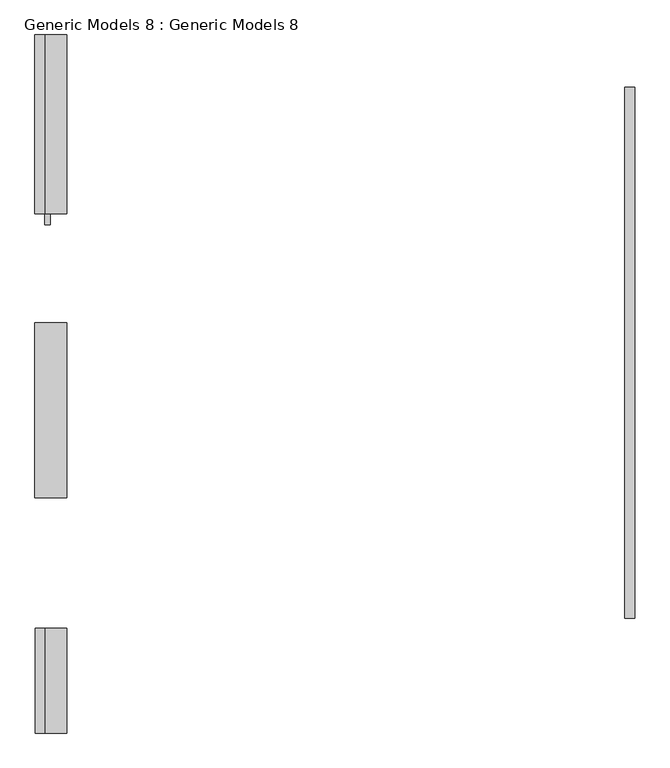
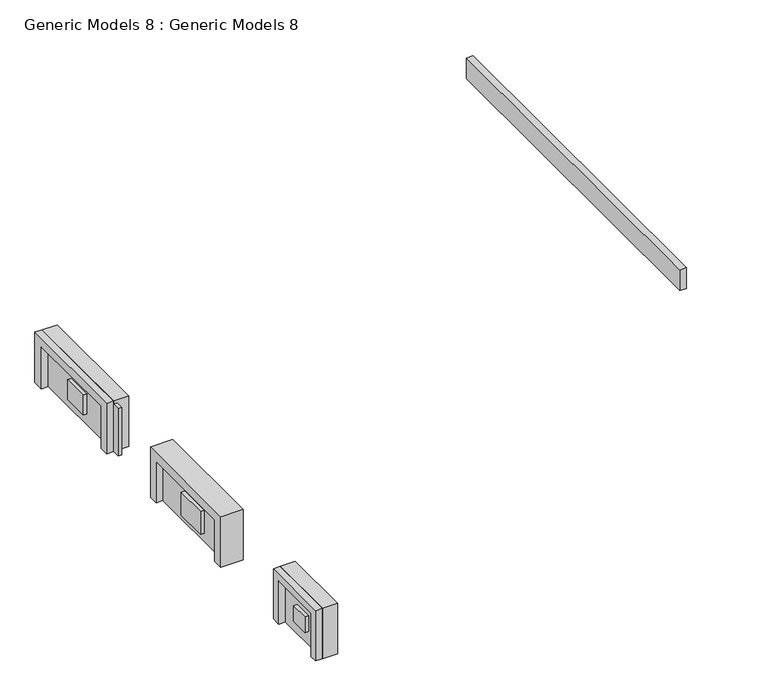
"""IFC4 building model written with IfcOpenShell, lengths in millimetres: proxy geometry, Generic Models 8 : Generic Models 8."""

from ifc_helpers import new_model, si_unit, frame, origin, origin_with_axes, place, context, project, spatial, polyline, outline, extrude, faceted_brep, source, transform, mapped, element, save


def generic_models_8_generic_models_8_478b8fa0(model_context):
    return source(origin(), model_context, "Body", "SolidModel", [
        extrude(outline(polyline([(-7844.1503587, -13644.7526331), (-7844.1503587, -1224.1526331), (-7615.5503587, -1224.1526331), (-7615.5503587, -13644.7526331), (-7844.1503587, -13644.7526331)])), frame((0.0, 0.0, 6400.8), z_axis=(0.0, 0.0, 1.0), x_axis=(1.0, 0.0, 0.0)), (0.0, 0.0, 1.0), 737.5181991),
        extrude(outline(polyline([(-21535.9206529, -15534.9751269), (-21535.9206529, -14874.5751269), (-21408.9206529, -14874.5751269), (-21408.9206529, -15534.9751269), (-21535.9206529, -15534.9751269)])), frame((0.0, 0.0, 181.195359), z_axis=(0.0, 0.0, 1.0), x_axis=(1.0, 0.0, 0.0)), (0.0, 0.0, 1.0), 558.8),
        extrude(outline(polyline([(-13873.3526331, -304.8), (-14178.4839562, -304.8), (-14178.4839562, 1232.1316532), (-16074.0892499, 1232.1316532), (-16074.0892499, -304.8), (-16330.8026331, -304.8), (-16330.8026331, 1483.4369838), (-13873.3526331, 1483.4369838), (-13873.3526331, -304.8)])), frame((-21637.5206529, 0.0, 0.0), z_axis=(1.0, 0.0, 0.0), x_axis=(0.0, 1.0, 0.0)), (0.0, 0.0, 1.0), 228.6),
        extrude(outline(polyline([(-21543.2828462, -9472.8026331), (-21543.2828462, -8342.5026331), (-21416.2828462, -8342.5026331), (-21416.2828462, -9472.8026331), (-21543.2828462, -9472.8026331)])), origin_with_axes(), (0.0, 0.0, 1.0), 812.6731894),
        faceted_brep([(-21644.8828462, -6729.6026331, -304.8), (-21644.8828462, -7051.784928, -304.8), (-21644.8828462, -7051.784928, 1165.4262933), (-21644.8828462, -10472.6342949, 1165.4262933), (-21644.8828462, -10472.6342949, -304.8), (-21644.8828462, -10825.3526331, -304.8), (-21644.8828462, -10825.3526331, 1483.4369838), (-21644.8828462, -6729.6026331, 1483.4369838), (-20900.9206529, -6729.6026331, -304.8), (-20900.9206529, -10825.3526331, -304.8), (-21416.2828462, -10472.6342949, -304.8), (-21416.2828462, -7051.784928, -304.8), (-21416.2828462, -7051.784928, 1165.4262933), (-20900.9206529, -10825.3526331, 1483.4369838), (-20900.9206529, -6729.6026331, 1483.4369838), (-21416.2828462, -10472.6342949, 1165.4262933)], [[[0, 1, 2, 3, 4, 5, 6, 7]], [[1, 0, 8, 9, 5, 4, 10, 11]], [[2, 1, 11, 12]], [[7, 6, 13, 14]], [[0, 7, 14, 8]], [[3, 2, 12, 15]], [[6, 5, 9, 13]], [[11, 10, 15, 12]], [[9, 8, 14, 13]], [[4, 3, 15, 10]]]),
        extrude(outline(polyline([(-21289.6793796, -4441.130528), (-21416.2828462, -4441.130528), (-21416.2828462, -4180.6282104), (-21289.6793796, -4180.6282104), (-21289.6793796, -4441.130528)])), frame((0.0, 0.0, -304.8), z_axis=(0.0, 0.0, 1.0), x_axis=(1.0, 0.0, 0.0)), (0.0, 0.0, 1.0), 1687.2104402),
        extrude(outline(polyline([(-21543.2828462, -2646.7809666), (-21543.2828462, -1732.3809666), (-21416.2828462, -1732.3809666), (-21416.2828462, -2646.7809666), (-21543.2828462, -2646.7809666)])), frame((0.0, 0.0, 101.4731894), z_axis=(0.0, 0.0, 1.0), x_axis=(1.0, 0.0, 0.0)), (0.0, 0.0, 1.0), 711.2),
        extrude(outline(polyline([(-0.5111724, -304.8), (-373.2526331, -304.8), (-373.2526331, 1189.7285902), (-3855.4970733, 1189.7285902), (-3855.4970733, -304.8), (-4180.6282104, -304.8), (-4180.6282104, 1483.4369838), (-0.5111724, 1483.4369838), (-0.5111724, -304.8)])), frame((-21644.8828462, 0.0, 0.0), z_axis=(1.0, 0.0, 0.0), x_axis=(0.0, 1.0, 0.0)), (0.0, 0.0, 1.0), 228.6),
        extrude(outline(polyline([(-21408.9206529, -16330.8026331), (-21408.9206529, -13873.3526331), (-20900.9206529, -13873.3526331), (-20900.9206529, -16330.8026331), (-21408.9206529, -16330.8026331)])), frame((0.0, 0.0, -304.8), z_axis=(0.0, 0.0, 1.0), x_axis=(1.0, 0.0, 0.0)), (0.0, 0.0, 1.0), 1788.2369838),
        extrude(outline(polyline([(-21416.2828462, -4180.6282104), (-21416.2828462, -0.5111724), (-20900.9206529, -0.5111724), (-20900.9206529, -4180.6282104), (-21416.2828462, -4180.6282104)])), frame((0.0, 0.0, -304.8), z_axis=(0.0, 0.0, 1.0), x_axis=(1.0, 0.0, 0.0)), (0.0, 0.0, 1.0), 1788.2369838),
    ])


if __name__ == "__main__":
    model = new_model("IFC4")
    model_context = context("Model", 3, world=origin())
    ifc_project = project(units=[si_unit("LENGTHUNIT", "METRE", prefix="MILLI")], contexts=[model_context])
    site = spatial("IfcSite", under=ifc_project)
    building = spatial("IfcBuilding", under=site)
    placement = place(None, origin())
    generic_models_8_generic_models_8_shape = generic_models_8_generic_models_8_478b8fa0(model_context)
    element("IfcBuildingElementProxy", 1, Name="Generic Models 8 : Generic Models 8", ObjectType="Generic Models 8 : Generic Models 8", at=placement, inside=building, context=model_context, shape_type="MappedRepresentation", body=[
        mapped(generic_models_8_generic_models_8_shape, transform((0.0, 0.0, 0.0), x_axis=(1.0, 0.0, 0.0), y_axis=(0.0, 1.0, 0.0), z_axis=(0.0, 0.0, 1.0))),
    ])
    save(model, "model.ifc")
